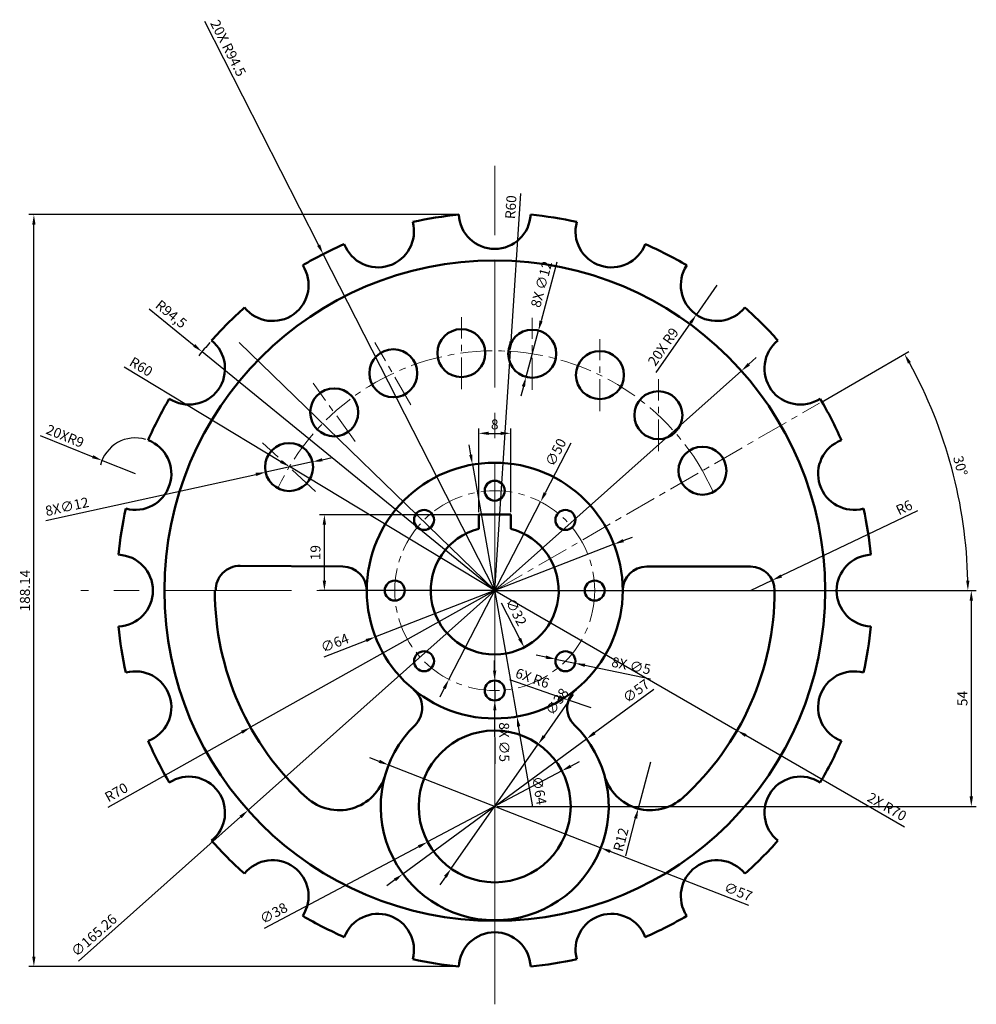
# Model space of a CAD drawing. Units: millimetres. Extents: x 2650 to 2889, y 1429 to 1675.
import ezdxf

# ---------------------------------------------------------------- set-up
doc = ezdxf.new("R2010")
doc.units = ezdxf.units.MM
doc.linetypes.add('CENTER', pattern=[50.8, 31.75, -6.35, 6.35, -6.35])
for name, color, linetype, lineweight in [('M-CNTR', 4, 'CENTER', 18), ('M-CONS', 8, 'Continuous', 13), ('M-DIMS', 2, 'Continuous', 25), ('M-OUTL', 7, 'Continuous', 50)]:
    doc.layers.add(name, color=color, linetype=linetype, lineweight=lineweight)
doc.styles.get("Standard").update_dxf_attribs({"font": 'arial.ttf'})
doc.dimstyles.new('ISO-25', dxfattribs={"dimtxt": 2.5, "dimasz": 2.5, "dimexe": 1.25, "dimexo": 0.625, "dimtad": 1, "dimtxsty": 'Standard', "dimcen": 2.5, "dimadec": 0, "dimazin": 0, "dimtfac": 1, "dimtmove": 0, "dimatfit": 3, "dimfxl": 1, "dimarcsym": 0})

# ---------------------------------------------------------------- blocks, each defined once
blk = doc.blocks.new('*D1')
at = {"layer": 'Defpoints', "color": 0, "transparency": 16777216}
for p in [(2726.24, 1551.15), (2768.85, 1551.15), (2768.85, 1532.15)]:
    blk.add_point(p, dxfattribs=at)
at = {"layer": 'M-DIMS', "color": 0, "lineweight": -2, "transparency": 16777216}
for p, q in [((2768.22, 1551.15), (2724.99, 1551.15)), ((2726.24, 1534.65), (2726.24, 1548.65)), ((2768.22, 1532.15), (2724.99, 1532.15))]:
    blk.add_line(p, q, dxfattribs=at)
at = {"layer": 'M-DIMS', "color": 0, "transparency": 16777216}
for points in [[(2725.82, 1548.65), (2726.66, 1548.65), (2726.24, 1551.15)], [(2725.82, 1534.65), (2726.66, 1534.65), (2726.24, 1532.15)]]:
    blk.add_solid(points, dxfattribs=at)
at = {"layer": 'M-DIMS', "color": 0, "transparency": 16777216, "insert": (2724.34, 1541.65), "char_height": 2.5, "attachment_point": 5, "rotation": 90}
blk.add_mtext('19', dxfattribs=at)
blk = doc.blocks.new('*D2')
at = {"layer": 'Defpoints', "color": 0, "transparency": 16777216}
for p in [(2772.85, 1571.5), (2764.85, 1551.15), (2772.85, 1551.15)]:
    blk.add_point(p, dxfattribs=at)
at = {"layer": 'M-DIMS', "color": 0, "lineweight": -2, "transparency": 16777216}
for p, q in [((2764.85, 1551.78), (2764.85, 1572.75)), ((2772.85, 1551.78), (2772.85, 1572.75)), ((2767.35, 1571.5), (2770.35, 1571.5))]:
    blk.add_line(p, q, dxfattribs=at)
at = {"layer": 'M-DIMS', "color": 0, "transparency": 16777216}
for points in [[(2767.35, 1571.92), (2767.35, 1571.09), (2764.85, 1571.5)], [(2770.35, 1571.92), (2770.35, 1571.09), (2772.85, 1571.5)]]:
    blk.add_solid(points, dxfattribs=at)
at = {"layer": 'M-DIMS', "color": 0, "transparency": 16777216, "insert": (2768.85, 1573.41), "char_height": 2.5, "attachment_point": 5}
blk.add_mtext('8', dxfattribs=at)
blk = doc.blocks.new('*D3')
at = {"layer": 'Defpoints', "color": 0, "transparency": 16777216}
for p in [(2838.26, 1534.74), (2832.85, 1532.15)]:
    blk.add_point(p, dxfattribs=at)
at = {"layer": 'M-DIMS', "color": 0, "lineweight": -2, "transparency": 16777216}
for p, q in [((2874.58, 1552.07), (2840.52, 1535.81)), ((2832.85, 1532.15), (2838.26, 1534.74))]:
    blk.add_line(p, q, dxfattribs=at)
at = {"layer": 'M-DIMS', "color": 0, "transparency": 16777216}
blk.add_solid([(2840.34, 1536.19), (2840.7, 1535.44), (2838.26, 1534.74)], dxfattribs=at)
at = {"layer": 'M-DIMS', "color": 0, "transparency": 16777216, "insert": (2871.38, 1552.65), "char_height": 2.5, "attachment_point": 5, "rotation": 25.5167}
blk.add_mtext('R6', dxfattribs=at)
blk = doc.blocks.new('*D4')
at = {"layer": 'Defpoints', "color": 0, "transparency": 16777216}
for p in [(2717.49, 1563.18), (2768.85, 1532.15)]:
    blk.add_point(p, dxfattribs=at)
at = {"layer": 'M-DIMS', "color": 0, "lineweight": -2, "transparency": 16777216}
for p, q in [((2676.17, 1588.14), (2715.35, 1564.47)), ((2768.85, 1532.15), (2717.49, 1563.18))]:
    blk.add_line(p, q, dxfattribs=at)
at = {"layer": 'M-DIMS', "color": 0, "transparency": 16777216}
blk.add_solid([(2715.57, 1564.83), (2715.13, 1564.11), (2717.49, 1563.18)], dxfattribs=at)
at = {"layer": 'M-DIMS', "color": 0, "transparency": 16777216, "insert": (2680.25, 1587.9), "char_height": 2.5, "attachment_point": 5, "rotation": 328.8637}
blk.add_mtext('R60', dxfattribs=at)
blk = doc.blocks.new('*D5')
at = {"layer": 'Defpoints', "color": 0, "transparency": 16777216}
for p in [(2695.64, 1591.91), (2768.85, 1532.15)]:
    blk.add_point(p, dxfattribs=at)
at = {"layer": 'M-DIMS', "color": 0, "lineweight": -2, "transparency": 16777216}
for p, q in [((2682.45, 1602.67), (2693.7, 1593.49)), ((2768.85, 1532.15), (2695.64, 1591.91))]:
    blk.add_line(p, q, dxfattribs=at)
blk.add_arc((2768.85, 1532.15), 94.5, 138.9201, 141.5365, dxfattribs=at)
at = {"layer": 'M-DIMS', "color": 0, "transparency": 16777216}
blk.add_solid([(2693.96, 1593.81), (2693.44, 1593.17), (2695.64, 1591.91)], dxfattribs=at)
at = {"layer": 'M-DIMS', "color": 0, "transparency": 16777216, "insert": (2687.73, 1601.1), "char_height": 2.5, "attachment_point": 5, "rotation": 320.7786}
blk.add_mtext('R94,5', dxfattribs=at)
blk = doc.blocks.new('*D6')
at = {"layer": 'Defpoints', "color": 0, "transparency": 16777216}
for p in [(2670.62, 1564.72), (2678.97, 1561.36)]:
    blk.add_point(p, dxfattribs=at)
at = {"layer": 'M-DIMS', "color": 0, "lineweight": -2, "transparency": 16777216}
for p, q in [((2655.16, 1570.95), (2668.3, 1565.65)), ((2678.97, 1561.36), (2670.62, 1564.72))]:
    blk.add_line(p, q, dxfattribs=at)
blk.add_arc((2678.97, 1561.36), 9, 73.2495, 166.0158, dxfattribs=at)
at = {"layer": 'M-DIMS', "color": 0, "transparency": 16777216}
blk.add_solid([(2668.46, 1566.04), (2668.15, 1565.27), (2670.62, 1564.72)], dxfattribs=at)
at = {"layer": 'M-DIMS', "color": 0, "transparency": 16777216, "insert": (2661.28, 1570.53), "char_height": 2.5, "attachment_point": 5, "rotation": 338.058}
blk.add_mtext('20XR9', dxfattribs=at)
blk = doc.blocks.new('*D7')
at = {"layer": 'Defpoints', "color": 0, "transparency": 16777216}
for p in [(2768.85, 1532.15), (2707.78, 1497.94)]:
    blk.add_point(p, dxfattribs=at)
at = {"layer": 'M-DIMS', "color": 0, "lineweight": -2, "transparency": 16777216}
for p, q in [((2768.85, 1532.15), (2707.78, 1497.94)), ((2672.16, 1477.98), (2705.6, 1496.72))]:
    blk.add_line(p, q, dxfattribs=at)
at = {"layer": 'M-DIMS', "color": 0, "transparency": 16777216}
blk.add_solid([(2705.39, 1497.08), (2705.8, 1496.35), (2707.78, 1497.94)], dxfattribs=at)
at = {"layer": 'M-DIMS', "color": 0, "transparency": 16777216, "insert": (2674.37, 1481.4), "char_height": 2.5, "attachment_point": 5, "rotation": 29.2611}
blk.add_mtext('R70', dxfattribs=at)
blk = doc.blocks.new('*D8')
at = {"layer": 'Defpoints', "color": 0, "transparency": 16777216}
for p in [(2807.81, 1489.19), (2804.73, 1477.59)]:
    blk.add_point(p, dxfattribs=at)
at = {"layer": 'M-DIMS', "color": 0, "lineweight": -2, "transparency": 16777216}
for p, q in [((2807.81, 1489.19), (2804.73, 1477.59)), ((2801.6, 1465.8), (2804.09, 1475.18))]:
    blk.add_line(p, q, dxfattribs=at)
at = {"layer": 'M-DIMS', "color": 0, "transparency": 16777216}
blk.add_solid([(2803.69, 1475.28), (2804.49, 1475.07), (2804.73, 1477.59)], dxfattribs=at)
at = {"layer": 'M-DIMS', "color": 0, "transparency": 16777216, "insert": (2800.71, 1469.77), "char_height": 2.5, "attachment_point": 5, "rotation": 75.1323}
blk.add_mtext('R12', dxfattribs=at)
blk = doc.blocks.new('*D9')
at = {"layer": 'Defpoints', "color": 0, "transparency": 16777216}
for p in [(2784.08, 1514.99), (2788.97, 1513.96)]:
    blk.add_point(p, dxfattribs=at)
at = {"layer": 'M-DIMS', "color": 0, "lineweight": -2, "transparency": 16777216}
for p, q in [((2781.63, 1515.5), (2779.18, 1516.01)), ((2784.08, 1514.99), (2788.97, 1513.96)), ((2807.84, 1510.01), (2791.42, 1513.45))]:
    blk.add_line(p, q, dxfattribs=at)
at = {"layer": 'M-DIMS', "color": 0, "transparency": 16777216}
for points in [[(2781.72, 1515.91), (2781.54, 1515.09), (2784.08, 1514.99)], [(2791.5, 1513.86), (2791.33, 1513.04), (2788.97, 1513.96)]]:
    blk.add_solid(points, dxfattribs=at)
at = {"layer": 'M-DIMS', "color": 0, "transparency": 16777216, "insert": (2802.92, 1513.05), "char_height": 2.5, "attachment_point": 5, "rotation": 348.1571}
blk.add_mtext('8X ∅5', dxfattribs=at)
blk = doc.blocks.new('*D10')
at = {"layer": 'Defpoints', "color": 0, "transparency": 16777216}
for p in [(2742.3, 1488.52), (2795.39, 1467.78)]:
    blk.add_point(p, dxfattribs=at)
at = {"layer": 'M-DIMS', "color": 0, "lineweight": -2, "transparency": 16777216}
for p, q in [((2739.97, 1489.43), (2737.64, 1490.34)), ((2742.3, 1488.52), (2795.39, 1467.78)), ((2832.43, 1453.32), (2797.72, 1466.87))]:
    blk.add_line(p, q, dxfattribs=at)
at = {"layer": 'M-DIMS', "color": 0, "transparency": 16777216}
for points in [[(2740.12, 1489.82), (2739.82, 1489.04), (2742.3, 1488.52)], [(2797.87, 1467.26), (2797.57, 1466.49), (2795.39, 1467.78)]]:
    blk.add_solid(points, dxfattribs=at)
at = {"layer": 'M-DIMS', "color": 0, "transparency": 16777216, "insert": (2829.63, 1456.53), "char_height": 2.5, "attachment_point": 5, "rotation": 338.666}
blk.add_mtext('∅57', dxfattribs=at)
blk = doc.blocks.new('*D11')
at = {"layer": 'Defpoints', "color": 0, "transparency": 16777216}
for p in [(2785.63, 1487.05), (2752.06, 1469.26)]:
    blk.add_point(p, dxfattribs=at)
at = {"layer": 'M-DIMS', "color": 0, "lineweight": -2, "transparency": 16777216}
for p, q in [((2787.84, 1488.22), (2790.05, 1489.39)), ((2785.63, 1487.05), (2752.06, 1469.26)), ((2711.29, 1447.65), (2749.85, 1468.08))]:
    blk.add_line(p, q, dxfattribs=at)
at = {"layer": 'M-DIMS', "color": 0, "transparency": 16777216}
for points in [[(2787.65, 1488.59), (2788.04, 1487.85), (2785.63, 1487.05)], [(2749.65, 1468.45), (2750.04, 1467.72), (2752.06, 1469.26)]]:
    blk.add_solid(points, dxfattribs=at)
at = {"layer": 'M-DIMS', "color": 0, "transparency": 16777216, "insert": (2713.71, 1451.16), "char_height": 2.5, "attachment_point": 5, "rotation": 27.9229}
blk.add_mtext('∅38', dxfattribs=at)
blk = doc.blocks.new('*D12')
at = {"layer": 'Defpoints', "color": 0, "transparency": 16777216}
for p in [(2798.67, 1543.75), (2739.02, 1520.56)]:
    blk.add_point(p, dxfattribs=at)
at = {"layer": 'M-DIMS', "color": 0, "lineweight": -2, "transparency": 16777216}
for p, q in [((2801, 1544.66), (2803.33, 1545.56)), ((2798.67, 1543.75), (2739.02, 1520.56)), ((2726.16, 1515.56), (2736.69, 1519.65))]:
    blk.add_line(p, q, dxfattribs=at)
at = {"layer": 'M-DIMS', "color": 0, "transparency": 16777216}
for points in [[(2800.85, 1545.04), (2801.15, 1544.27), (2798.67, 1543.75)], [(2736.54, 1520.04), (2736.84, 1519.26), (2739.02, 1520.56)]]:
    blk.add_solid(points, dxfattribs=at)
at = {"layer": 'M-DIMS', "color": 0, "transparency": 16777216, "insert": (2728.96, 1518.76), "char_height": 2.5, "attachment_point": 5, "rotation": 21.2469}
blk.add_mtext('∅64', dxfattribs=at)
blk = doc.blocks.new('*D13')
at = {"layer": 'Defpoints', "color": 0, "transparency": 16777216}
for p in [(2780.31, 1554.37), (2757.38, 1509.94)]:
    blk.add_point(p, dxfattribs=at)
at = {"layer": 'M-DIMS', "color": 0, "lineweight": -2, "transparency": 16777216}
for p, q in [((2787.89, 1569.06), (2781.46, 1556.59)), ((2757.38, 1509.94), (2780.31, 1554.37)), ((2756.24, 1507.71), (2755.09, 1505.49))]:
    blk.add_line(p, q, dxfattribs=at)
at = {"layer": 'M-DIMS', "color": 0, "transparency": 16777216}
for points in [[(2781.08, 1556.78), (2781.83, 1556.4), (2780.31, 1554.37)], [(2755.87, 1507.9), (2756.61, 1507.52), (2757.38, 1509.94)]]:
    blk.add_solid(points, dxfattribs=at)
at = {"layer": 'M-DIMS', "color": 0, "transparency": 16777216, "insert": (2784.4, 1566.61), "char_height": 2.5, "attachment_point": 5, "rotation": 62.7094}
blk.add_mtext('∅50', dxfattribs=at)
blk = doc.blocks.new('*D14')
at = {"layer": 'Defpoints', "color": 0, "transparency": 16777216}
for p in [(2723.28, 1564.35), (2711.56, 1561.77)]:
    blk.add_point(p, dxfattribs=at)
at = {"layer": 'M-DIMS', "color": 0, "lineweight": -2, "transparency": 16777216}
for p, q in [((2725.72, 1564.88), (2728.16, 1565.42)), ((2723.28, 1564.35), (2711.56, 1561.77)), ((2656.61, 1549.67), (2709.12, 1561.23))]:
    blk.add_line(p, q, dxfattribs=at)
at = {"layer": 'M-DIMS', "color": 0, "transparency": 16777216}
for points in [[(2725.63, 1565.29), (2725.81, 1564.48), (2723.28, 1564.35)], [(2709.03, 1561.63), (2709.2, 1560.82), (2711.56, 1561.77)]]:
    blk.add_solid(points, dxfattribs=at)
at = {"layer": 'M-DIMS', "color": 0, "transparency": 16777216, "insert": (2661.95, 1552.86), "char_height": 2.5, "attachment_point": 5, "rotation": 12.4152}
blk.add_mtext('8X∅12', dxfattribs=at)
blk = doc.blocks.new('*D15')
at = {"layer": 'Defpoints', "color": 0, "transparency": 16777216}
for p in [(2761.49, 1546.36), (2776.21, 1517.95)]:
    blk.add_point(p, dxfattribs=at)
at = {"layer": 'M-DIMS', "color": 0, "lineweight": -2, "transparency": 16777216}
blk.add_line((2770.44, 1529.07), (2775.06, 1520.17), dxfattribs=at)
at = {"layer": 'M-DIMS', "color": 0, "transparency": 16777216}
blk.add_solid([(2775.43, 1520.36), (2774.69, 1519.97), (2776.21, 1517.95)], dxfattribs=at)
at = {"layer": 'M-DIMS', "color": 0, "transparency": 16777216, "insert": (2773.93, 1526.63), "char_height": 2.5, "attachment_point": 5, "rotation": 297.3914}
blk.add_mtext('∅32', dxfattribs=at)
blk = doc.blocks.new('*D16')
at = {"layer": 'Defpoints', "color": 0, "transparency": 16777216}
for p in [(2850.03, 1579.03), (2885.38, 1552.7), (2768.85, 1532.15), (2768.85, 1532.15), (2885.05, 1532.15)]:
    blk.add_point(p, dxfattribs=at)
at = {"layer": 'M-DIMS', "color": 0, "lineweight": -2, "transparency": 16777216}
for p, q in [((2850.58, 1579.34), (2872.41, 1591.95)), ((2885.68, 1532.15), (2888.43, 1532.15))]:
    blk.add_line(p, q, dxfattribs=at)
blk.add_arc((2768.85, 1532.15), 118.34, 1.2105, 28.7895, dxfattribs=at)
at = {"layer": 'M-DIMS', "color": 0, "transparency": 16777216}
for points in [[(2872.19, 1588.94), (2872.92, 1589.35), (2871.33, 1591.32)], [(2887.57, 1534.66), (2886.74, 1534.65), (2887.18, 1532.15)]]:
    blk.add_solid(points, dxfattribs=at)
at = {"layer": 'M-DIMS', "color": 0, "transparency": 16777216, "insert": (2884.99, 1563.27), "char_height": 2.5, "attachment_point": 5, "rotation": 285}
blk.add_mtext('30°', dxfattribs=at)
blk = doc.blocks.new('*D17')
at = {"layer": 'Defpoints', "color": 0, "transparency": 16777216}
for p in [(2768.85, 1532.15), (2768.85, 1478.15), (2888.04, 1478.15)]:
    blk.add_point(p, dxfattribs=at)
at = {"layer": 'M-DIMS', "color": 0, "lineweight": -2, "transparency": 16777216}
for p, q in [((2769.47, 1532.15), (2889.29, 1532.15)), ((2888.04, 1529.65), (2888.04, 1480.65)), ((2769.47, 1478.15), (2889.29, 1478.15))]:
    blk.add_line(p, q, dxfattribs=at)
at = {"layer": 'M-DIMS', "color": 0, "transparency": 16777216}
for points in [[(2887.62, 1529.65), (2888.45, 1529.65), (2888.04, 1532.15)], [(2887.62, 1480.65), (2888.45, 1480.65), (2888.04, 1478.15)]]:
    blk.add_solid(points, dxfattribs=at)
at = {"layer": 'M-DIMS', "color": 0, "transparency": 16777216, "insert": (2886.14, 1505.15), "char_height": 2.5, "attachment_point": 5, "rotation": 90}
blk.add_mtext('54', dxfattribs=at)
blk = doc.blocks.new('PLATE-HOLE-D12')
blk.add_circle((6, 6), 6)
blk = doc.blocks.new('HUB-HOLE-D5')
blk.add_circle((2.5, 2.5), 2.5)
blk = doc.blocks.new('*D20')
at = {"layer": 'Defpoints', "color": 0, "transparency": 16777216}
for p in [(2653.59, 1626.22), (2759.86, 1626.22), (2759.86, 1438.08)]:
    blk.add_point(p, dxfattribs=at)
at = {"layer": 'M-DIMS', "color": 0, "lineweight": -2, "transparency": 16777216}
for p, q in [((2759.23, 1626.22), (2652.34, 1626.22)), ((2653.59, 1440.58), (2653.59, 1623.72)), ((2759.23, 1438.08), (2652.34, 1438.08))]:
    blk.add_line(p, q, dxfattribs=at)
at = {"layer": 'M-DIMS', "color": 0, "transparency": 16777216}
for points in [[(2653.17, 1623.72), (2654, 1623.72), (2653.59, 1626.22)], [(2653.17, 1440.58), (2654, 1440.58), (2653.59, 1438.08)]]:
    blk.add_solid(points, dxfattribs=at)
at = {"layer": 'M-DIMS', "color": 0, "transparency": 16777216, "insert": (2651.68, 1532.15), "char_height": 2.5, "attachment_point": 5, "rotation": 90}
blk.add_mtext('188.14', dxfattribs=at)
blk = doc.blocks.new('*D21')
at = {"layer": 'Defpoints', "color": 0, "transparency": 16777216}
for p in [(2725.94, 1616.35), (2768.85, 1532.15)]:
    blk.add_point(p, dxfattribs=at)
at = {"layer": 'M-DIMS', "color": 0, "lineweight": -2, "transparency": 16777216}
for p, q in [((2696.23, 1674.67), (2724.81, 1618.58)), ((2768.85, 1532.15), (2725.94, 1616.35))]:
    blk.add_line(p, q, dxfattribs=at)
at = {"layer": 'M-DIMS', "color": 0, "transparency": 16777216}
blk.add_solid([(2725.18, 1618.77), (2724.44, 1618.39), (2725.94, 1616.35)], dxfattribs=at)
at = {"layer": 'M-DIMS', "color": 0, "transparency": 16777216, "insert": (2701.9, 1667.74), "char_height": 2.5, "attachment_point": 5, "rotation": 297.0001}
blk.add_mtext('20X R94.5', dxfattribs=at)
blk = doc.blocks.new('*D22')
at = {"layer": 'Defpoints', "color": 0, "transparency": 16777216}
for p in [(2824.39, 1608.61), (2819.27, 1601.21)]:
    blk.add_point(p, dxfattribs=at)
at = {"layer": 'M-DIMS', "color": 0, "lineweight": -2, "transparency": 16777216}
for p, q in [((2824.39, 1608.61), (2819.27, 1601.21)), ((2809.23, 1586.7), (2817.85, 1599.15))]:
    blk.add_line(p, q, dxfattribs=at)
at = {"layer": 'M-DIMS', "color": 0, "transparency": 16777216}
blk.add_solid([(2817.5, 1599.39), (2818.19, 1598.91), (2819.27, 1601.21)], dxfattribs=at)
at = {"layer": 'M-DIMS', "color": 0, "transparency": 16777216, "insert": (2811.26, 1592.98), "char_height": 2.5, "attachment_point": 5, "rotation": 55.307}
blk.add_mtext('20X R9', dxfattribs=at)
blk = doc.blocks.new('*D23')
at = {"layer": 'Defpoints', "color": 0, "transparency": 16777216}
for p in [(2830.54, 1587.12), (2707.15, 1477.18)]:
    blk.add_point(p, dxfattribs=at)
at = {"layer": 'M-DIMS', "color": 0, "lineweight": -2, "transparency": 16777216}
for p, q in [((2832.41, 1588.79), (2834.27, 1590.45)), ((2830.54, 1587.12), (2707.15, 1477.18)), ((2664.78, 1439.43), (2705.29, 1475.52))]:
    blk.add_line(p, q, dxfattribs=at)
at = {"layer": 'M-DIMS', "color": 0, "transparency": 16777216}
for points in [[(2832.13, 1589.1), (2832.68, 1588.47), (2830.54, 1587.12)], [(2705.01, 1475.83), (2705.56, 1475.21), (2707.15, 1477.18)]]:
    blk.add_solid(points, dxfattribs=at)
at = {"layer": 'M-DIMS', "color": 0, "transparency": 16777216, "insert": (2668.83, 1445.67), "char_height": 2.5, "attachment_point": 5, "rotation": 41.7018}
blk.add_mtext('∅165.26', dxfattribs=at)
blk = doc.blocks.new('*D24')
at = {"layer": 'Defpoints', "color": 0, "transparency": 16777216}
for p in [(2768.85, 1532.15), (2829.47, 1497.15)]:
    blk.add_point(p, dxfattribs=at)
at = {"layer": 'M-DIMS', "color": 0, "lineweight": -2, "transparency": 16777216}
for p, q in [((2768.85, 1532.15), (2829.47, 1497.15)), ((2871.31, 1473), (2831.63, 1495.9))]:
    blk.add_line(p, q, dxfattribs=at)
at = {"layer": 'M-DIMS', "color": 0, "transparency": 16777216}
blk.add_solid([(2831.84, 1496.26), (2831.43, 1495.54), (2829.47, 1497.15)], dxfattribs=at)
at = {"layer": 'M-DIMS', "color": 0, "transparency": 16777216, "insert": (2866.79, 1477.8), "char_height": 2.5, "attachment_point": 5, "rotation": 330.0004}
blk.add_mtext('2X R70', dxfattribs=at)
blk = doc.blocks.new('*D25')
at = {"layer": 'Defpoints', "color": 0, "transparency": 16777216}
for p in [(2772.75, 1592.03), (2768.85, 1532.15)]:
    blk.add_point(p, dxfattribs=at)
at = {"layer": 'M-DIMS', "color": 0, "lineweight": -2, "transparency": 16777216}
for p, q in [((2775.33, 1631.55), (2772.91, 1594.52)), ((2768.85, 1532.15), (2772.75, 1592.03))]:
    blk.add_line(p, q, dxfattribs=at)
at = {"layer": 'M-DIMS', "color": 0, "transparency": 16777216}
blk.add_solid([(2772.5, 1594.55), (2773.33, 1594.49), (2772.75, 1592.03)], dxfattribs=at)
at = {"layer": 'M-DIMS', "color": 0, "transparency": 16777216, "insert": (2773.19, 1628.07), "char_height": 2.5, "attachment_point": 5, "rotation": 86.2697}
blk.add_mtext('R60', dxfattribs=at)
blk = doc.blocks.new('*D26')
at = {"layer": 'Defpoints', "color": 0, "transparency": 16777216}
for p in [(2763.29, 1563.67), (2774.4, 1500.64)]:
    blk.add_point(p, dxfattribs=at)
at = {"layer": 'M-DIMS', "color": 0, "lineweight": -2, "transparency": 16777216}
for p, q in [((2762.86, 1566.13), (2762.42, 1568.59)), ((2763.29, 1563.67), (2774.4, 1500.64)), ((2778.39, 1478.02), (2774.83, 1498.18))]:
    blk.add_line(p, q, dxfattribs=at)
at = {"layer": 'M-DIMS', "color": 0, "transparency": 16777216}
for points in [[(2763.27, 1566.2), (2762.45, 1566.06), (2763.29, 1563.67)], [(2775.24, 1498.25), (2774.42, 1498.1), (2774.4, 1500.64)]]:
    blk.add_solid(points, dxfattribs=at)
at = {"layer": 'M-DIMS', "color": 0, "transparency": 16777216, "insert": (2779.67, 1482.07), "char_height": 2.5, "attachment_point": 5, "rotation": 279.9945}
blk.add_mtext('∅64', dxfattribs=at)
blk = doc.blocks.new('*D27')
at = {"layer": 'Defpoints', "color": 0, "transparency": 16777216}
for p in [(2791.8, 1495.05), (2745.89, 1461.26)]:
    blk.add_point(p, dxfattribs=at)
at = {"layer": 'M-DIMS', "color": 0, "lineweight": -2, "transparency": 16777216}
for p, q in [((2808.61, 1507.42), (2793.81, 1496.53)), ((2745.89, 1461.26), (2791.8, 1495.05)), ((2743.88, 1459.78), (2741.87, 1458.3))]:
    blk.add_line(p, q, dxfattribs=at)
at = {"layer": 'M-DIMS', "color": 0, "transparency": 16777216}
for points in [[(2793.57, 1496.86), (2794.06, 1496.19), (2791.8, 1495.05)], [(2743.63, 1460.11), (2744.13, 1459.44), (2745.89, 1461.26)]]:
    blk.add_solid(points, dxfattribs=at)
at = {"layer": 'M-DIMS', "color": 0, "transparency": 16777216, "insert": (2804.4, 1506.77), "char_height": 2.5, "attachment_point": 5, "rotation": 36.3534}
blk.add_mtext('∅57', dxfattribs=at)
blk = doc.blocks.new('*D28')
at = {"layer": 'Defpoints', "color": 0, "transparency": 16777216}
for p in [(2779.74, 1493.72), (2757.95, 1462.59)]:
    blk.add_point(p, dxfattribs=at)
at = {"layer": 'M-DIMS', "color": 0, "lineweight": -2, "transparency": 16777216}
for p, q in [((2788.45, 1506.15), (2781.18, 1495.77)), ((2757.95, 1462.59), (2779.74, 1493.72)), ((2756.52, 1460.54), (2755.08, 1458.49))]:
    blk.add_line(p, q, dxfattribs=at)
at = {"layer": 'M-DIMS', "color": 0, "transparency": 16777216}
for points in [[(2780.84, 1496), (2781.52, 1495.53), (2779.74, 1493.72)], [(2756.17, 1460.78), (2756.86, 1460.3), (2757.95, 1462.59)]]:
    blk.add_solid(points, dxfattribs=at)
at = {"layer": 'M-DIMS', "color": 0, "transparency": 16777216, "insert": (2784.67, 1504.19), "char_height": 2.5, "attachment_point": 5, "rotation": 55.0029}
blk.add_mtext('∅38', dxfattribs=at)
blk = doc.blocks.new('*D29')
at = {"layer": 'Defpoints', "color": 0, "transparency": 16777216}
for p in [(2787.31, 1504.76), (2792.98, 1502.8)]:
    blk.add_point(p, dxfattribs=at)
at = {"layer": 'M-DIMS', "color": 0, "lineweight": -2, "transparency": 16777216}
for p, q in [((2772.51, 1509.89), (2784.95, 1505.58)), ((2792.98, 1502.8), (2787.31, 1504.76))]:
    blk.add_line(p, q, dxfattribs=at)
at = {"layer": 'M-DIMS', "color": 0, "transparency": 16777216}
blk.add_solid([(2785.09, 1505.98), (2784.81, 1505.19), (2787.31, 1504.76)], dxfattribs=at)
at = {"layer": 'M-DIMS', "color": 0, "transparency": 16777216, "insert": (2778.17, 1509.94), "char_height": 2.5, "attachment_point": 5, "rotation": 340.9206}
blk.add_mtext('6X R6', dxfattribs=at)
blk = doc.blocks.new('*D30')
at = {"layer": 'Defpoints', "color": 0, "transparency": 16777216}
for p in [(2779.79, 1597.21), (2776.68, 1585.62)]:
    blk.add_point(p, dxfattribs=at)
at = {"layer": 'M-DIMS', "color": 0, "lineweight": -2, "transparency": 16777216}
for p, q in [((2784.39, 1614.37), (2780.43, 1599.62)), ((2776.68, 1585.62), (2779.79, 1597.21)), ((2776.03, 1583.2), (2775.38, 1580.79))]:
    blk.add_line(p, q, dxfattribs=at)
at = {"layer": 'M-DIMS', "color": 0, "transparency": 16777216}
for points in [[(2780.03, 1599.73), (2780.84, 1599.52), (2779.79, 1597.21)], [(2775.63, 1583.31), (2776.43, 1583.1), (2776.68, 1585.62)]]:
    blk.add_solid(points, dxfattribs=at)
at = {"layer": 'M-DIMS', "color": 0, "transparency": 16777216, "insert": (2780.83, 1608.72), "char_height": 2.5, "attachment_point": 5, "rotation": 74.9945}
blk.add_mtext('8X ∅12', dxfattribs=at)
blk = doc.blocks.new('*D31')
at = {"layer": 'Defpoints', "color": 0, "transparency": 16777216}
for p in [(2768.83, 1509.65), (2768.86, 1504.65)]:
    blk.add_point(p, dxfattribs=at)
at = {"layer": 'M-DIMS', "color": 0, "lineweight": -2, "transparency": 16777216}
for p, q in [((2768.82, 1512.15), (2768.81, 1514.65)), ((2768.83, 1509.65), (2768.86, 1504.65)), ((2768.95, 1488.78), (2768.87, 1502.15))]:
    blk.add_line(p, q, dxfattribs=at)
at = {"layer": 'M-DIMS', "color": 0, "transparency": 16777216}
for points in [[(2769.24, 1512.16), (2768.4, 1512.15), (2768.83, 1509.65)], [(2769.29, 1502.16), (2768.46, 1502.15), (2768.86, 1504.65)]]:
    blk.add_solid(points, dxfattribs=at)
at = {"layer": 'M-DIMS', "color": 0, "transparency": 16777216, "insert": (2770.89, 1494.23), "char_height": 2.5, "attachment_point": 5, "rotation": 270.3128}
blk.add_mtext('8X ∅5', dxfattribs=at)

msp = doc.modelspace()

# ---------------------------------------------------------------- linework, layer by layer
at = {"layer": 'M-CNTR'}
for p, q in [((2768.846, 1625.496), (2768.846, 1638.445)), ((2768.846, 1532.153), (2768.846, 1625.496)), ((2768.846, 1532.153), (2665.336, 1532.153)), ((2768.846, 1532.153), (2768.846, 1456.552)), ((2768.846, 1532.153), (2885.051, 1532.153)), ((2768.846, 1456.552), (2768.846, 1428.636))]:
    msp.add_line(p, q, dxfattribs=at)
at = {"layer": 'M-CNTR', "ltscale": 0.25}
for p, q in [((2760.496, 1582.569), (2760.496, 1600.569)), ((2778.232, 1582.414), (2778.232, 1600.414)), ((2747.847, 1578.657), (2738.849, 1594.243)), ((2795.149, 1577.081), (2795.149, 1595.081)), ((2809.766, 1567.034), (2809.766, 1585.034)), ((2733.961, 1569.44), (2723.436, 1584.043)), ((2768.846, 1532.153), (2850.035, 1579.027)), ((2724.041, 1556.963), (2710.792, 1569.148)), ((2820.808, 1562.153), (2823.531, 1556.806))]:
    msp.add_line(p, q, dxfattribs=at)
msp.add_circle((2768.846, 1532.153), 25, dxfattribs=at)
msp.add_arc((2768.846, 1532.153), 60, 30, 154.73197, dxfattribs=at)
at = {"layer": 'M-CONS'}
for p, q in [((2768.846, 1532.153), (2704.922, 1594.192)), ((2768.846, 1532.153), (2768.846, 1551.153)), ((2736.846, 1532.153), (2730.846, 1532.153)), ((2768.846, 1532.153), (2768.846, 1478.153))]:
    msp.add_line(p, q, dxfattribs=at)
at = {"layer": 'M-OUTL'}
for p, q in [((2768.846, 1551.153), (2764.846, 1551.153)), ((2764.846, 1551.153), (2764.846, 1547.645)), ((2768.846, 1551.153), (2772.846, 1551.153)), ((2772.846, 1551.153), (2772.846, 1547.645)), ((2705.081, 1538.337), (2730.889, 1538.153)), ((2806.846, 1538.153), (2832.846, 1538.153))]:
    msp.add_line(p, q, dxfattribs=at)
for centre, radius in [((2768.846, 1532.153), 82.629), ((2717.416, 1563.055), 6), ((2768.846, 1532.153), 32), ((2786.524, 1514.475), 2.5), ((2768.846, 1478.153), 19)]:
    msp.add_circle(centre, radius, dxfattribs=at)
for centre, radius, start, end in [((2768.846, 1532.153), 94.5, 95.45881, 102.54119), ((2768.846, 1626.653), 9, 182.7294, 357.2706), ((2768.846, 1532.153), 94.5, 77.45881, 84.54119), ((2739.644, 1622.028), 9, 200.7294, 15.2706), ((2798.048, 1622.028), 9, 164.7294, 339.2706), ((2768.846, 1532.153), 94.5, 113.45881, 120.54119), ((2768.846, 1532.153), 94.5, 59.45881, 66.54119), ((2713.301, 1608.605), 9, 218.7294, 33.2706), ((2824.392, 1608.605), 9, 146.7294, 321.2706), ((2768.846, 1532.153), 94.5, 131.45881, 138.54119), ((2768.846, 1532.153), 94.5, 41.45881, 48.54119), ((2692.394, 1587.699), 9, 236.7294, 51.2706), ((2845.298, 1587.699), 9, 128.7294, 303.2706), ((2768.846, 1532.153), 94.5, 149.45881, 156.54119), ((2768.846, 1532.153), 94.5, 23.45881, 30.54119), ((2678.972, 1561.355), 9, 254.7294, 69.2706), ((2858.721, 1561.355), 9, 110.7294, 285.2706), ((2768.846, 1532.153), 94.5, 167.45881, 174.54119), ((2768.846, 1532.153), 94.5, 5.45881, 12.54119), ((2768.846, 1532.153), 16, 104.47751, 75.52249), ((2674.346, 1532.153), 9, 272.7294, 87.2706), ((2863.346, 1532.153), 9, 92.7294, 267.2706), ((2705.081, 1532.337), 6, 89.1818, 181.75855), ((2730.846, 1532.153), 6, 0, 89.5909), ((2806.846, 1532.153), 6, 90, 180), ((2832.846, 1532.153), 6, 0, 90), ((2768.846, 1532.153), 70, 180, 227.79115), ((2768.846, 1532.153), 70, 312.20885, 0), ((2768.846, 1532.153), 94.5, 185.45881, 192.54119), ((2768.846, 1532.153), 94.5, 347.45881, 354.54119), ((2678.972, 1502.951), 9, 290.7294, 105.2706), ((2858.721, 1502.951), 9, 74.7294, 249.2706), ((2744.709, 1502.803), 6, 314.39726, 50.56595), ((2792.984, 1502.803), 6, 129.43405, 225.60274), ((2768.846, 1478.153), 28.5, 134.39726, 45.60274), ((2768.846, 1532.153), 94.5, 203.45881, 210.54119), ((2768.846, 1532.153), 94.5, 329.45881, 336.54119), ((2692.394, 1476.607), 9, 308.7294, 123.2706), ((2729.88, 1489.192), 12, 227.79115, 344.18235), ((2807.813, 1489.192), 12, 195.81765, 312.20885), ((2845.298, 1476.607), 9, 56.7294, 231.2706), ((2768.846, 1532.153), 94.5, 221.45881, 228.54119), ((2768.846, 1532.153), 94.5, 311.45881, 318.54119), ((2713.301, 1455.701), 9, 326.7294, 141.2706), ((2824.392, 1455.701), 9, 38.7294, 213.2706), ((2739.644, 1442.278), 9, 344.7294, 159.2706), ((2798.048, 1442.278), 9, 20.7294, 195.2706), ((2768.846, 1532.153), 94.5, 239.45881, 246.54119), ((2768.846, 1532.153), 94.5, 293.45881, 300.54119), ((2768.846, 1437.653), 9, 2.7294, 177.2706), ((2768.846, 1532.153), 94.5, 257.45881, 264.54119), ((2768.846, 1532.153), 94.5, 275.45881, 282.54119)]:
    msp.add_arc(centre, radius, start, end, dxfattribs=at)

# ---------------------------------------------------------------- block references
for name, p in [('PLATE-HOLE-D12', (2754.496, 1585.569)), ('PLATE-HOLE-D12', (2772.233, 1585.414)), ('PLATE-HOLE-D12', (2737.489, 1580.531)), ('PLATE-HOLE-D12', (2789.149, 1580.081)), ('PLATE-HOLE-D12', (2722.699, 1570.742)), ('PLATE-HOLE-D12', (2803.766, 1570.034)), ('PLATE-HOLE-D12', (2814.808, 1556.153)), ('HUB-HOLE-D5', (2766.346, 1554.653)), ('HUB-HOLE-D5', (2748.668, 1547.331)), ('HUB-HOLE-D5', (2784.024, 1547.331)), ('HUB-HOLE-D5', (2741.346, 1529.653)), ('HUB-HOLE-D5', (2791.346, 1529.653)), ('HUB-HOLE-D5', (2748.668, 1511.975)), ('HUB-HOLE-D5', (2766.346, 1504.653))]:
    msp.add_blockref(name, p, dxfattribs=at)

# ---------------------------------------------------------------- dimensions: what is measured, and where the dimension line sits
at = {"layer": 'M-DIMS'}
for mpoint, text, override, picture, middle in [((2725.944, 1616.353), '20X <>', {"dimdec": 1, "dimlfac": 1, "dimrnd": 0, "dimzin": 0, "dimdsep": 46, "dimlunit": 2}, '*D21', (2700.203, 1666.873)), ((2829.468, 1497.153), '2X <>', {"dimdec": 0, "dimlfac": 1, "dimrnd": 0, "dimzin": 0, "dimdsep": 46, "dimlunit": 2}, '*D24', (2865.842, 1476.154))]:
    dim = msp.add_radius_dim(center=(2768.846, 1532.153), mpoint=mpoint, text=text, dimstyle='ISO-25', override=override, dxfattribs=at)
    dim.commit()
    dim.dimension.update_dxf_attribs({"geometry": picture, "text_midpoint": middle, "dimtype": 164})
for center, mpoint, override, picture, middle in [((2768.846, 1532.153), (2772.75, 1592.026), {"dimdec": 0, "dimlfac": 1, "dimrnd": 0, "dimzin": 0, "dimdsep": 46, "dimlunit": 2}, '*D25', (2775.092, 1627.95)), ((2768.846, 1532.153), (2695.636, 1591.907), {"dimclrd": 0, "dimclre": 0, "dimclrt": 0}, '*D5', (2686.389, 1599.455)), ((2768.846, 1532.153), (2717.49, 1563.177), {"dimclrd": 0, "dimclre": 0, "dimclrt": 0}, '*D4', (2679.262, 1586.271)), ((2832.846, 1532.153), (2838.261, 1534.738), {"dimclrd": 0, "dimclre": 0, "dimclrt": 0}, '*D3', (2872.199, 1550.937)), ((2768.846, 1532.153), (2707.778, 1497.938), {"dimclrd": 0, "dimclre": 0, "dimclrt": 0}, '*D7', (2675.303, 1479.743))]:
    dim = msp.add_radius_dim(center=center, mpoint=mpoint, dimstyle='ISO-25', override=override, dxfattribs=at)
    dim.commit()
    dim.dimension.update_dxf_attribs({"geometry": picture, "text_midpoint": middle, "dimtype": 164})
for base, p1, p2, override, picture, middle in [((2653.586, 1626.224), (2759.857, 1438.081), (2759.857, 1626.224), {"dimdec": 2, "dimlfac": 1, "dimrnd": 0, "dimzin": 0, "dimdsep": 46, "dimlunit": 2}, '*D20', (2651.684, 1532.153)), ((2726.241, 1551.153), (2768.846, 1532.153), (2768.846, 1551.153), {"dimclrd": 0, "dimclre": 0, "dimclrt": 0}, '*D1', (2724.34, 1541.653)), ((2888.035, 1478.153), (2768.846, 1532.153), (2768.846, 1478.153), {"dimclrd": 0, "dimclre": 0, "dimclrt": 0}, '*D17', (2886.139, 1505.153))]:
    dim = msp.add_linear_dim(base=base, p1=p1, p2=p2, angle=90, dimstyle='ISO-25', override=override, dxfattribs=at)
    dim.commit()
    dim.dimension.update_dxf_attribs({"geometry": picture, "text_midpoint": middle})
for p1, p2, text, override, picture, middle in [((2776.679, 1585.619), (2779.786, 1597.21), '8X <>', {"dimdec": 0, "dimlfac": 1, "dimrnd": 0, "dimzin": 0, "dimdsep": 46, "dimlunit": 2}, '*D30', (2782.733, 1608.205)), ((2723.276, 1564.345), (2711.557, 1561.765), '8X<>', {"dimclrd": 0, "dimclre": 0, "dimclrt": 0}, '*D14', (2662.37, 1550.937)), ((2784.077, 1514.988), (2788.971, 1513.962), '8X <>', {"dimclrd": 0, "dimclre": 0, "dimclrt": 0}, '*D9', (2802.52, 1511.121))]:
    dim = msp.add_diameter_dim_2p(p1=p1, p2=p2, text=text, dimstyle='ISO-25', override=override, dxfattribs=at)
    dim.commit()
    dim.dimension.update_dxf_attribs({"geometry": picture, "text_midpoint": middle, "dimtype": 163})
for center, mpoint, text, override, picture, middle in [((2824.392, 1608.605), (2819.269, 1601.205), '20X <>', {"dimdec": 0, "dimlfac": 1, "dimrnd": 0, "dimzin": 0, "dimdsep": 46, "dimlunit": 2}, '*D22', (2811.262, 1592.979)), ((2678.972, 1561.355), (2670.623, 1564.718), '20X<>', {"dimclrd": 0, "dimclre": 0, "dimclrt": 0}, '*D6', (2661.282, 1570.531)), ((2792.984, 1502.803), (2787.313, 1504.765), '6X <>', {"dimdec": 0, "dimlfac": 1, "dimrnd": 0, "dimzin": 0, "dimdsep": 46, "dimlunit": 2}, '*D29', (2778.17, 1509.939))]:
    dim = msp.add_radius_dim(center=center, mpoint=mpoint, text=text, dimstyle='ISO-25', override=override, dxfattribs=at)
    dim.commit()
    dim.dimension.update_dxf_attribs({"geometry": picture, "text_midpoint": middle})
dim = msp.add_angular_dim_2l(base=(2885.385, 1552.702), line1=((2768.846, 1532.153), (2885.051, 1532.153)), line2=((2768.846, 1532.153), (2850.035, 1579.027)), dimstyle='ISO-25', override={"dimclrd": 0, "dimclre": 0, "dimclrt": 0}, dxfattribs=at)
dim.commit()
dim.dimension.update_dxf_attribs({"geometry": '*D16', "text_midpoint": (2884.988, 1563.273)})
for p1, p2, override, picture, middle in [((2830.539, 1587.122), (2707.154, 1477.183), {"dimdec": 2, "dimlfac": 1, "dimrnd": 0, "dimzin": 0, "dimdsep": 46, "dimlunit": 2}, '*D23', (2670.138, 1444.202)), ((2757.384, 1509.936), (2780.309, 1554.37), {"dimclrd": 0, "dimclre": 0, "dimclrt": 0}, '*D13', (2786.156, 1565.704)), ((2763.293, 1563.667), (2774.4, 1500.639), {"dimdec": 0, "dimlfac": 1, "dimrnd": 0, "dimzin": 0, "dimdsep": 46, "dimlunit": 2}, '*D26', (2777.732, 1481.73)), ((2798.671, 1543.749), (2739.021, 1520.556), {"dimclrd": 0, "dimclre": 0, "dimclrt": 0}, '*D12', (2729.674, 1516.922)), ((2761.485, 1546.359), (2776.207, 1517.947), {"dimclrd": 0, "dimclre": 0, "dimclrt": 0}, '*D15', (2772.176, 1525.727)), ((2745.893, 1461.259), (2791.8, 1495.047), {"dimdec": 0, "dimlfac": 1, "dimrnd": 0, "dimzin": 0, "dimdsep": 46, "dimlunit": 2}, '*D27', (2805.571, 1505.183)), ((2757.949, 1462.588), (2779.744, 1493.717), {"dimdec": 0, "dimlfac": 1, "dimrnd": 0, "dimzin": 0, "dimdsep": 46, "dimlunit": 2}, '*D28', (2786.282, 1503.056)), ((2785.634, 1487.05), (2752.058, 1469.256), {"dimclrd": 0, "dimclre": 0, "dimclrt": 0}, '*D11', (2714.63, 1449.419)), ((2742.299, 1488.521), (2795.393, 1467.784), {"dimclrd": 0, "dimclre": 0, "dimclrt": 0}, '*D10', (2828.914, 1454.693))]:
    dim = msp.add_diameter_dim_2p(p1=p1, p2=p2, dimstyle='ISO-25', override=override, dxfattribs=at)
    dim.commit()
    dim.dimension.update_dxf_attribs({"geometry": picture, "text_midpoint": middle, "dimtype": 163})
dim = msp.add_linear_dim(base=(2772.846, 1571.505), p1=(2764.846, 1551.153), p2=(2772.846, 1551.153), dimstyle='ISO-25', override={"dimclrd": 0, "dimclre": 0, "dimclrt": 0}, dxfattribs=at)
dim.commit()
dim.dimension.update_dxf_attribs({"geometry": '*D2', "text_midpoint": (2768.846, 1573.406)})
dim = msp.add_diameter_dim_2p(p1=(2768.833, 1509.653), p2=(2768.86, 1504.653), text='8X <>', dimstyle='ISO-25', override={"dimdec": 0, "dimlfac": 1, "dimrnd": 0, "dimzin": 0, "dimdsep": 46, "dimlunit": 2}, dxfattribs=at)
dim.commit()
dim.dimension.update_dxf_attribs({"geometry": '*D31', "text_midpoint": (2768.917, 1494.218)})
dim = msp.add_radius_dim(center=(2807.813, 1489.192), mpoint=(2804.734, 1477.594), dimstyle='ISO-25', override={"dimclrd": 0, "dimclre": 0, "dimclrt": 0}, dxfattribs=at)
dim.commit()
dim.dimension.update_dxf_attribs({"geometry": '*D8', "text_midpoint": (2800.71, 1469.765)})

doc.saveas('drawing.dxf')
